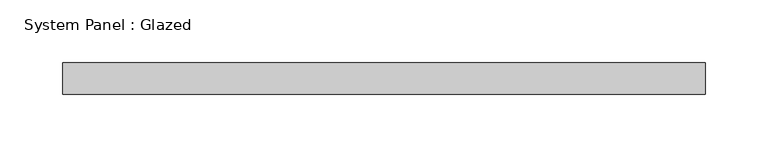
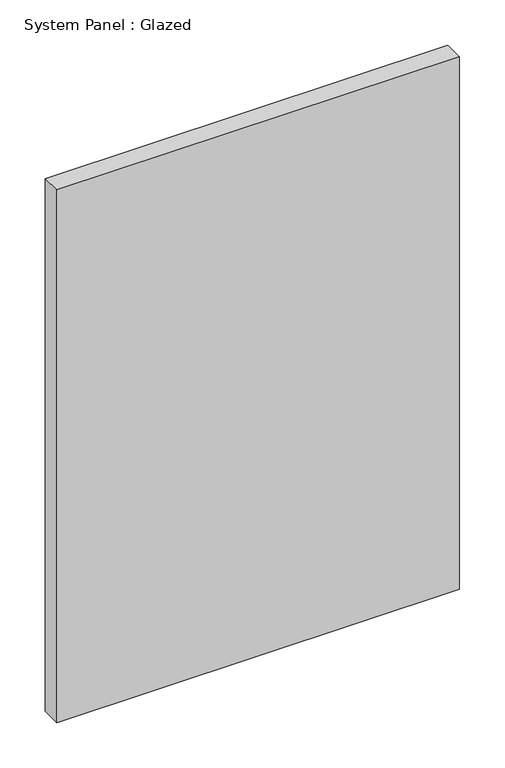
"""IFC4 building model written with IfcOpenShell, lengths in millimetres: plate geometry, System Panel : Glazed."""

from ifc_helpers import new_model, si_unit, origin, origin_with_axes, place, context, project, spatial, polyline, outline, extrude, source, transform, mapped, element, save


def system_panel_glazed_7650606a(model_context):
    return source(origin(), model_context, "Body", "SweptSolid", [
        extrude(outline(polyline([(257.175, 19.05), (-257.175, 19.05), (-257.175, 44.45), (257.175, 44.45), (257.175, 19.05)])), origin_with_axes(), (0.0, 0.0, 1.0), 719.3261324),
    ])


if __name__ == "__main__":
    model = new_model("IFC4")
    model_context = context("Model", 3, world=origin())
    ifc_project = project(units=[si_unit("LENGTHUNIT", "METRE", prefix="MILLI")], contexts=[model_context])
    site = spatial("IfcSite", under=ifc_project)
    building = spatial("IfcBuilding", under=site)
    placement = place(None, origin())
    system_panel_glazed_shape = system_panel_glazed_7650606a(model_context)
    element("IfcPlate", 1, ObjectType="System Panel : Glazed", at=placement, inside=building, context=model_context, shape_type="MappedRepresentation", body=[
        mapped(system_panel_glazed_shape, transform((0.0, 0.0, 0.0), x_axis=(1.0, 0.0, 0.0), y_axis=(0.0, 1.0, 0.0), z_axis=(0.0, 0.0, 1.0))),
    ])
    save(model, "model.ifc")

# Revit data of these elements
# Type "System Panel : Glazed"
#   Construction Type Id = "GSP4R"
#   Analytic Construction = "1/8 in Pilkington single glazing"
#   Visual Light Transmittance = 0.9
#   Solar Heat Gain Coefficient = 0.86
#   Heat Transfer Coefficient (U) = 1.18115 BTU/(h·ft²·°F)
#   Define Thermal Properties by = 1
# Element 1 (IfcPlate, "System Panel : Glazed")
#   Materials on its faces: "Glass"
# Materials
#   "Glass": class "Glass", colour RGB 0 128 192, transparency 0.75, Description = "Soda Lime Glass", Cost = 0
